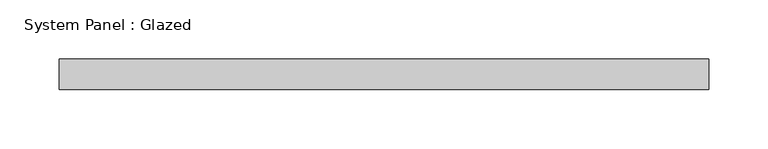
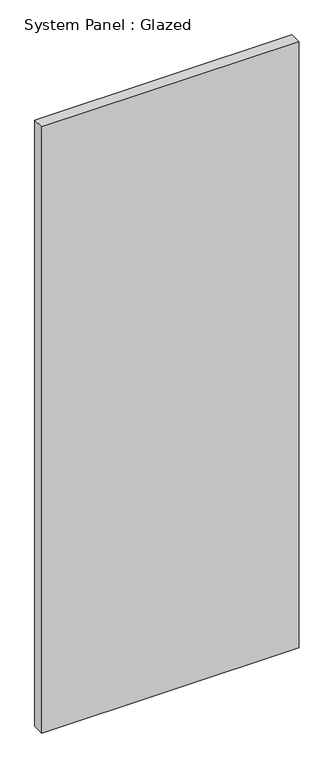
"""IFC4 building model written with IfcOpenShell, lengths in millimetres: plate geometry, System Panel : Glazed."""

from ifc_helpers import new_model, si_unit, origin, origin_with_axes, place, context, project, spatial, polyline, outline, extrude, source, transform, mapped, element, save


def system_panel_glazed_42028690(model_context):
    return source(origin(), model_context, "Body", "SweptSolid", [
        extrude(outline(polyline([(273.05, 19.05), (-273.05, 19.05), (-273.05, 44.45), (273.05, 44.45), (273.05, 19.05)])), origin_with_axes(), (0.0, 0.0, 1.0), 1359.7688321),
    ])


if __name__ == "__main__":
    model = new_model("IFC4")
    model_context = context("Model", 3, world=origin())
    ifc_project = project(units=[si_unit("LENGTHUNIT", "METRE", prefix="MILLI")], contexts=[model_context])
    site = spatial("IfcSite", under=ifc_project)
    building = spatial("IfcBuilding", under=site)
    placement = place(None, origin())
    system_panel_glazed_shape = system_panel_glazed_42028690(model_context)
    element("IfcPlate", 1, ObjectType="System Panel : Glazed", at=placement, inside=building, context=model_context, shape_type="MappedRepresentation", body=[
        mapped(system_panel_glazed_shape, transform((0.0, 0.0, 0.0), x_axis=(1.0, 0.0, 0.0), y_axis=(0.0, 1.0, 0.0), z_axis=(0.0, 0.0, 1.0))),
    ])
    save(model, "model.ifc")

# Revit data of these elements
# Type "System Panel : Glazed"
#   Construction Type Id = "GSP4R"
#   Analytic Construction = "1/8 in Pilkington single glazing"
#   Visual Light Transmittance = 0.9
#   Solar Heat Gain Coefficient = 0.86
#   Heat Transfer Coefficient (U) = 1.18115 BTU/(h·ft²·°F)
#   Define Thermal Properties by = 1
# Element 1 (IfcPlate, "System Panel : Glazed")
#   Materials on its faces: "Glass"
# Materials
#   "Glass": class "Glass", colour RGB 0 128 192, transparency 0.75, Description = "Soda Lime Glass", Cost = 0
